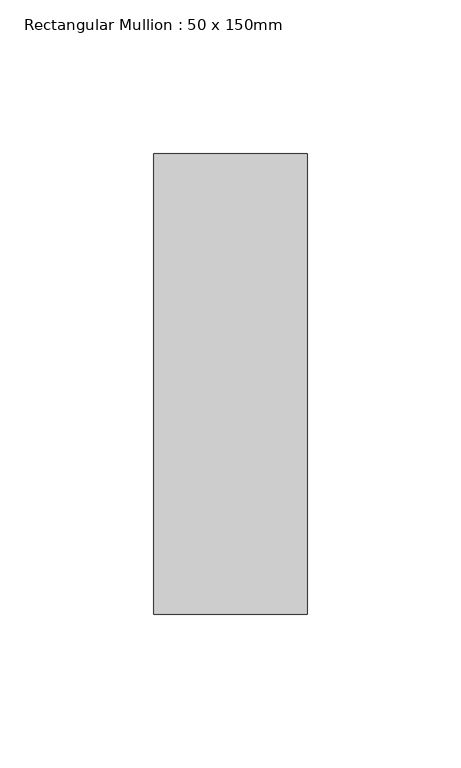
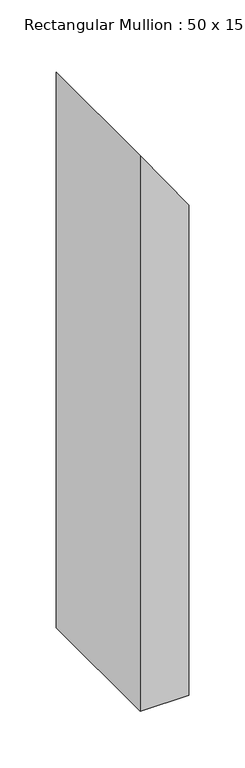
"""IFC4 building model written with IfcOpenShell, lengths in millimetres: member geometry, Rectangular Mullion : 50 x 150mm."""

from ifc_helpers import new_model, si_unit, frame, origin, place, context, project, spatial, polyline, outline, extrude, source, transform, mapped, element, save


def rectangular_mullion_50_x_150mm_bd832bbd(model_context):
    return source(origin(), model_context, "Body", "SweptSolid", [
        extrude(outline(polyline([(-122.8760399, 25.0), (-51.4686396, -25.0), (-657.4074958, -25.0), (-657.4074958, 25.0), (-122.8760399, 25.0)])), frame((0.0, -75.0, 0.0), z_axis=(0.0, 1.0, 0.0), x_axis=(0.0, 0.0, 1.0)), (0.0, 0.0, 1.0), 150.0),
    ])


if __name__ == "__main__":
    model = new_model("IFC4")
    model_context = context("Model", 3, world=origin())
    ifc_project = project(units=[si_unit("LENGTHUNIT", "METRE", prefix="MILLI")], contexts=[model_context])
    site = spatial("IfcSite", under=ifc_project)
    building = spatial("IfcBuilding", under=site)
    placement = place(None, origin())
    rectangular_mullion_50_x_150mm_shape = rectangular_mullion_50_x_150mm_bd832bbd(model_context)
    element("IfcMember", 1, ObjectType="Rectangular Mullion : 50 x 150mm", at=placement, inside=building, context=model_context, shape_type="MappedRepresentation", body=[
        mapped(rectangular_mullion_50_x_150mm_shape, transform((0.0, 0.0, 0.0), x_axis=(1.0, 0.0, 0.0), y_axis=(0.0, 1.0, 0.0), z_axis=(0.0, 0.0, 1.0))),
    ])
    save(model, "model.ifc")

# Revit data of these elements
# Type "Rectangular Mullion : 50 x 150mm"
#   built-in parameter 1007304 = 0.492126 (stored number, unit not read)
#   built-in parameter 1007301 = 0.082021 (stored number, unit not read)
#   built-in parameter 1007300 = 0.082021 (stored number, unit not read)
# Element 1 (IfcMember, "Rectangular Mullion : 50 x 150mm")
#   Materials on its faces: "Aluminium"
# Materials
#   "Aluminium": class "Metal", colour RGB 247 247 247, transparency 0, Description = "Aluminium 6061", Cost = 0
